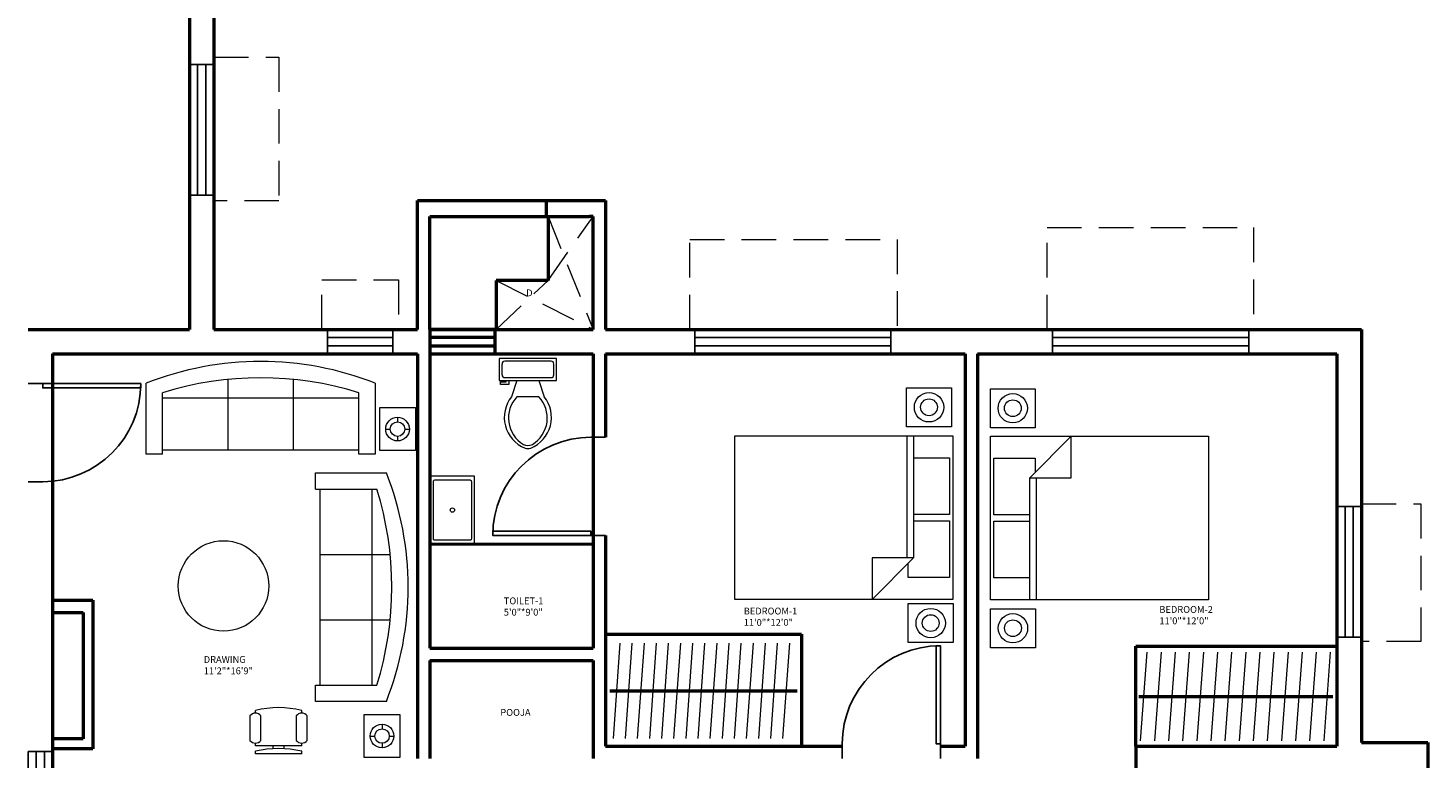
# Model space of a CAD drawing. Units: inches. Extents: x 291 to 2631, y 456 to 2623.
# Tile 11 of 22: x 2109 to 2623, y 774 to 1042. Entities that reach past the tile are written whole.
import ezdxf

# ---------------------------------------------------------------- set-up
doc = ezdxf.new("R2010")
doc.units = ezdxf.units.IN
doc.linetypes.add('DASHED', pattern=[19.05, 12.7, -6.35])
for name, color, linetype, lineweight in [('A-ANNO-TEXT', 3, 'Continuous', 25), ('A-AREA-IDEN', 7, 'Continuous', 25), ('A-DOOR', 3, 'Continuous', 25), ('A-FLOR-FIXT', 9, 'Continuous', 18), ('A-FLOR-OVHD', 1, 'DASHED', 18), ('A-FURN', 8, 'Continuous', 18), ('A-GLAZ', 4, 'Continuous', 25), ('A-WALL', 7, 'Continuous', 50)]:
    doc.layers.add(name, color=color, linetype=linetype, lineweight=lineweight)
doc.styles.get("Standard").update_dxf_attribs({"font": 'arial.ttf'})

# ---------------------------------------------------------------- blocks, each defined once
blk = doc.blocks.new('*U2')
for p, q in [((0, 0), (0, -6)), ((40, 0), (40, -6))]:
    blk.add_line(p, q)
blk.add_lwpolyline([(0, 0), (0, 40), (1.75, 40), (1.75, 0)], close=True)
blk.add_arc((0, 0), 40, 0, 90)
blk = doc.blocks.new('Sofa - Roundback 7 ft.')
for p, q in [((-12.00002, -32.4421), (-12.00003, -6.5971)), ((11.99997, -32.4421), (11.99998, -6.5971)), ((-36.000027, -34), (-36.000027, -11.4696)), ((-35.999844, -13.3819), (35.9998, -13.3819)), ((35.99998, -34), (35.99998, -11.4696)), ((-36.000027, -32.4421), (35.99998, -32.4421))]:
    blk.add_line(p, q)
for points in [[(-36.000027, -34), (-42.000027, -34), (-42.000027, -8)], [(41.99998, -8), (41.99998, -34), (35.99998, -34)]]:
    blk.add_lwpolyline(points)
for centre, radius, start, end in [((0, -114.25), 114.25, 68.43141, 111.5686), ((-0.00001, -127.1968), 121.1968, 72.72033, 107.2797)]:
    blk.add_arc(centre, radius, start, end)
blk = doc.blocks.new('Chair - Desk')
for p, q in [((-8.5, 0), (-8.5, -1)), ((-8.5, 0), (8.5, 0)), ((8.5, 0), (8.5, -1)), ((-10.5, -5), (-10.5, -14)), ((-8.5, -3), (-8.5, -4)), ((-8.5, -3), (8.5, -3)), ((-6.5, -14), (-6.5, -5)), ((-2, -3), (-2, -1.9355)), ((2, -1.9576), (2, -3)), ((6.5, -5), (6.5, -14)), ((8.5, -3), (8.5, -4)), ((10.5, -14), (10.5, -5)), ((-8.5, -15), (-8.5, -16)), ((8.5, -15), (8.5, -16))]:
    blk.add_line(p, q)
for centre, radius, start, end in [((-8.5, -6.5), 2.5, 36.8699, 143.1301), ((0, 34.625), 36.625, 256.5803, 283.4197), ((8.5, -6.5), 2.5, 36.8699, 143.1301), ((-8.5, -12.5), 2.5, 216.8699, 323.1301), ((8.5, -12.5), 2.5, 216.8699, 323.1301), ((0, 19.625), 36.625, 256.5803, 283.4197)]:
    blk.add_arc(centre, radius, start, end)
blk = doc.blocks.new('Toilet - top')
for p, q in [((9.5, -6), (9.5, -2)), ((-10, -8.5), (-8, -8.5)), ((-10, -9.5), (-10, -8.5)), ((-7, -9.5), (-10, -9.5)), ((-8, -8.5), (-8, -8)), ((-7, -8), (-7, -9.5)), ((-4, -8), (-6, -14)), ((4, -8), (6, -14)), ((4, -14), (-4, -14))]:
    blk.add_line(p, q)
blk.add_lwpolyline([(10.5, -8), (10.5, 0), (-10.5, 0), (-10.5, -8)], close=True)
for points in [[(-9.5, -2), (-9.5, -6)], [(8.5, -1), (-8.5, -1)], [(-8.5, -7), (8.5, -7)]]:
    blk.add_lwpolyline(points)
for centre, radius, start, end in [((-8.62, -1.88), 0.884, 81.8699, 188.1301), ((8.62, -1.88), 0.884, 351.8699, 98.1301), ((-8.62, -6.12), 0.884, 171.8699, 278.1301), ((8.62, -6.12), 0.884, 261.8699, 8.1301), ((3.52, -21.58), 12.17, 141.4691, 247.9714), ((4.2, -21.82), 11.33, 136.3677, 238.9468), ((-3.52, -21.58), 12.17, 292.0284, 38.5307), ((-4.2, -21.82), 11.33, 301.053, 43.6321), ((0, -27.88), 4, 245.7318, 294.2682), ((0, -29), 4, 254.8605, 285.1395)]:
    blk.add_arc(centre, radius, start, end)
blk = doc.blocks.new('Bed - Queen')
for p, q in [((0, -80.00003), (0, 0)), ((0, 0), (59.99999, 0)), ((59.99999, 0), (59.99999, -80.00003)), ((7.99999, -1.2), (28.79998, -1.2)), ((7.99999, -14.4), (7.99999, -1.2)), ((28.79998, -1.2), (28.79998, -14.4)), ((31.19999, -1.2), (51.99999, -1.2)), ((31.19999, -14.4), (31.19999, -1.2)), ((51.99999, -1.2), (51.99999, -16.4)), ((0, -14.4), (44.8, -14.4)), ((59.99999, -29.6), (44.8, -14.4)), ((44.8, -14.4), (44.8, -29.6)), ((44.8, -16.8), (0, -16.8)), ((51.99999, -16.4), (46.79936, -16.4)), ((44.8, -29.6), (59.99999, -29.6)), ((59.99999, -80.00003), (0, -80.00003))]:
    blk.add_line(p, q)
blk = doc.blocks.new('WIN-1800')
for p, q in [((0, 9), (72, 9)), ((0, 0), (0, 9)), ((0, 6), (72, 6)), ((72, 9), (72, 0)), ((72, 3), (0, 3)), ((72, 0), (0, 0))]:
    blk.add_line(p, q)
blk = doc.blocks.new('WIN-1200')
for p, q in [((0, 0), (0, 48)), ((0, 48), (9, 48)), ((3, 0), (3, 48)), ((6, 48), (6, 0)), ((9, 48), (9, 0)), ((9, 0), (0, 0))]:
    blk.add_line(p, q)
blk = doc.blocks.new('WIN-600')
for p, q in [((24, 9), (0, 9)), ((0, 9), (0, 0)), ((24, 6), (0, 6)), ((24, 0), (24, 9)), ((0, 3), (24, 3)), ((0, 0), (24, 0))]:
    blk.add_line(p, q)
blk = doc.blocks.new('LAMP-A')
for p, q in [((6.55, 12.25), (6.55, 10.56)), ((2.2, 7.9), (3.88, 7.9)), ((6.55, 5.24), (6.55, 3.56)), ((9.21, 7.9), (10.89, 7.9))]:
    blk.add_line(p, q)
blk.add_lwpolyline([(0, 15.8), (13.09, 15.8), (13.09, 0), (0, 0)], close=True)
for radius in [4.34, 2.66]:
    blk.add_circle((6.55, 7.9), radius)

msp = doc.modelspace()

# ---------------------------------------------------------------- linework, layer by layer
at = {"layer": 'A-FLOR-OVHD'}
for p, q in [((2177.21, 1030.97), (2201.09, 1030.97)), ((2201.09, 1030.97), (2201.09, 978.24)), ((2201.09, 978.24), (2177.21, 978.24)), ((2299.87, 972.51), (2316.47, 930.98)), ((2299.87, 948.94), (2316.47, 972.51)), ((2483.05, 930.98), (2483.05, 968.4)), ((2483.05, 968.4), (2558.88, 968.4)), ((2558.88, 968.4), (2558.88, 930.98)), ((2351.9, 930.98), (2351.9, 964.04)), ((2351.9, 964.04), (2428.07, 964.04)), ((2428.07, 964.04), (2428.07, 930.98)), ((2216.81, 930.98), (2216.81, 949.22)), ((2216.81, 949.22), (2244.97, 949.22)), ((2244.97, 949.22), (2244.97, 930.98)), ((2280.82, 948.94), (2316.47, 930.98)), ((2280.82, 930.98), (2299.87, 948.94)), ((2598.47, 866.98), (2620.33, 866.98)), ((2620.33, 866.98), (2620.33, 816.39)), ((2620.33, 816.39), (2598.47, 816.39))]:
    msp.add_line(p, q, dxfattribs=at)
at = {"layer": 'A-FURN'}
for p, q in [((2323.87, 780.85), (2326.34, 815.77)), ((2328.32, 780.85), (2330.78, 815.77)), ((2332.76, 780.85), (2335.23, 815.77)), ((2337.21, 780.85), (2339.68, 815.77)), ((2341.66, 780.85), (2344.12, 815.77)), ((2346.1, 780.85), (2348.57, 815.77)), ((2350.55, 780.85), (2353.02, 815.77)), ((2355, 780.85), (2357.46, 815.77)), ((2359.44, 780.85), (2361.91, 815.77)), ((2363.89, 780.85), (2366.35, 815.77)), ((2368.33, 780.85), (2370.8, 815.77)), ((2372.78, 780.85), (2375.25, 815.77)), ((2377.23, 780.85), (2379.69, 815.77)), ((2381.67, 780.85), (2384.14, 815.77)), ((2386.12, 780.85), (2388.59, 815.77)), ((2517.42, 779.97), (2519.86, 812.55)), ((2522.6, 779.97), (2525.04, 812.55)), ((2527.77, 779.97), (2530.22, 812.55)), ((2532.95, 779.97), (2535.4, 812.55)), ((2538.13, 779.97), (2540.57, 812.55)), ((2543.31, 779.97), (2545.75, 812.55)), ((2548.48, 779.97), (2550.93, 812.55)), ((2553.66, 779.97), (2556.11, 812.55)), ((2558.84, 779.97), (2561.28, 812.55)), ((2564.02, 779.97), (2566.46, 812.55)), ((2569.2, 779.97), (2571.64, 812.55)), ((2574.37, 779.97), (2576.82, 812.55)), ((2579.55, 779.97), (2581.99, 812.55)), ((2584.73, 779.97), (2587.17, 812.55))]:
    msp.add_line(p, q, dxfattribs=at)
for points in [[(2431.49, 909.56), (2447.97, 909.56), (2447.97, 895.26), (2431.49, 895.26)], [(2462.24, 909.21), (2478.72, 909.21), (2478.72, 894.91), (2462.24, 894.91)], [(2256.47, 852.14), (2272.82, 852.14), (2272.82, 877.08), (2256.47, 877.08)], [(2432.11, 830.34), (2448.59, 830.34), (2448.59, 816.04), (2432.11, 816.04)], [(2462.3, 828.43), (2478.78, 828.43), (2478.78, 814.13), (2462.3, 814.13)]]:
    msp.add_lwpolyline(points, close=True, dxfattribs=at)
msp.add_lwpolyline([(2258.32, 875.72), (2271.24, 875.72, -0.414214), (2271.74, 875.22), (2271.74, 854.12, -0.414214), (2271.24, 853.62), (2258.32, 853.62, -0.414214), (2257.82, 854.12), (2257.82, 875.22, -0.414214)], format="xyb", close=True, dxfattribs=at)
for centre, radius in [((2439.73, 902.41), 5.39), ((2439.73, 902.41), 3.08), ((2470.48, 902.06), 5.39), ((2470.48, 902.06), 3.08), ((2264.78, 864.67), 0.806), ((2180.72, 836.81), 16.61), ((2440.35, 823.19), 5.39), ((2440.35, 823.19), 3.08), ((2470.54, 821.28), 5.39), ((2470.54, 821.28), 3.08)]:
    msp.add_circle(centre, radius, dxfattribs=at)
at = {"layer": 'A-WALL'}
for p, q in [((2168.21, 1112.52), (2168.21, 930.98)), ((2177.21, 1112.52), (2177.21, 930.98)), ((2251.97, 930.98), (2251.97, 978.3)), ((2251.97, 978.3), (2320.97, 978.3)), ((2299.15, 978.3), (2299.15, 972.51)), ((2320.97, 978.3), (2320.97, 930.98)), ((2256.47, 930.98), (2256.47, 972.51)), ((2256.47, 972.51), (2314.97, 972.51)), ((2299.87, 972.51), (2299.87, 948.94)), ((2316.47, 972.51), (2314.97, 972.51)), ((2316.47, 930.98), (2316.47, 972.51)), ((2299.87, 948.94), (2280.82, 948.94)), ((2280.82, 948.94), (2280.82, 930.98)), ((2108.97, 930.98), (2168.21, 930.98)), ((2177.21, 930.98), (2251.97, 930.98)), ((2256.47, 930.98), (2256.47, 813.98)), ((2280.47, 930.98), (2256.47, 930.98)), ((2256.47, 930.98), (2256.47, 921.98)), ((2256.47, 930.98), (2316.47, 930.98)), ((2280.47, 921.98), (2280.47, 930.98)), ((2320.97, 930.98), (2598.47, 930.98)), ((2598.47, 930.98), (2598.47, 779.28)), ((2280.47, 927.98), (2256.47, 927.98)), ((2117.97, 921.98), (2251.97, 921.98)), ((2117.97, 921.98), (2117.97, 720.98)), ((2251.97, 921.98), (2251.97, 773.48)), ((2256.47, 924.98), (2280.47, 924.98)), ((2256.47, 921.98), (2280.47, 921.98)), ((2256.47, 921.98), (2316.47, 921.98)), ((2316.47, 921.98), (2316.47, 813.98)), ((2320.97, 921.98), (2320.97, 891.39)), ((2320.97, 921.98), (2452.97, 921.98)), ((2452.97, 921.98), (2452.97, 777.98)), ((2457.47, 921.98), (2457.47, 773.48)), ((2457.47, 921.98), (2589.47, 921.98)), ((2589.47, 921.98), (2589.47, 777.98)), ((2320.97, 855.39), (2320.97, 777.98)), ((2256.47, 852.14), (2316.47, 852.23)), ((2117.97, 831.6), (2132.79, 831.6)), ((2132.79, 831.6), (2132.79, 777.06)), ((2117.97, 827.07), (2129.19, 827.07)), ((2129.19, 827.07), (2129.19, 780.66)), ((2320.97, 819.07), (2392.97, 819.07)), ((2392.97, 819.07), (2392.97, 777.98)), ((2256.47, 813.98), (2316.47, 813.98)), ((2515.69, 777.98), (2515.69, 814.67)), ((2515.69, 814.67), (2589.47, 814.67)), ((2256.47, 809.48), (2316.47, 809.48)), ((2256.47, 809.48), (2256.47, 773.48)), ((2316.47, 809.48), (2316.47, 773.48)), ((2322.5, 798.31), (2391.31, 798.31)), ((2516.78, 796.26), (2587.92, 796.26)), ((2129.19, 780.66), (2117.97, 780.66)), ((2132.79, 777.06), (2117.97, 777.06)), ((2320.97, 777.98), (2407.89, 777.98)), ((2443.89, 777.98), (2452.97, 777.98)), ((2515.69, 777.98), (2515.69, 765.67)), ((2515.69, 777.98), (2589.47, 777.98)), ((2598.47, 779.28), (2621.78, 779.28)), ((2621.78, 779.28), (2622.9, 779.28)), ((2622.9, 779.28), (2622.9, 756.88))]:
    msp.add_line(p, q, dxfattribs=at)

# ---------------------------------------------------------------- block references
at = {"layer": 'A-DOOR', "xscale": 0.9, "yscale": 0.9, "zscale": 0.9}
for p, rotation in [((2114.37, 911.1), 270), ((2315.57, 855.39), 90)]:
    msp.add_blockref('*U2', p, dxfattribs=dict(at, rotation=rotation))
at = {"layer": 'A-DOOR', "xscale": -0.9, "yscale": 0.9, "zscale": 0.9}
msp.add_blockref('*U2', (2443.89, 778.88), dxfattribs=at)
at = {"layer": 'A-FLOR-FIXT'}
msp.add_blockref('Toilet - top', (2292.47, 920.3), dxfattribs=at)
at = {"layer": 'A-FURN'}
for name, p in [('Sofa - Roundback 7 ft.', (2194.4, 919.24)), ('LAMP-A', (2238.07, 886.5)), ('LAMP-A', (2232.38, 773.82))]:
    msp.add_blockref(name, p, dxfattribs=at)
for name, p, rotation in [('Bed - Queen', (2448.46, 891.9), 270), ('Bed - Queen', (2462.29, 831.75), 90), ('Sofa - Roundback 7 ft.', (2248.52, 836.39), 270), ('Chair - Desk', (2200.94, 775.13), 180)]:
    msp.add_blockref(name, p, dxfattribs=dict(at, rotation=rotation))
at = {"layer": 'A-GLAZ', "rotation": 180}
for name, p in [('WIN-1200', (2177.21, 1028.26)), ('WIN-600', (2242.87, 930.98)), ('WIN-1200', (2598.47, 865.99)), ('WIN-1200', (2117.97, 776.04))]:
    msp.add_blockref(name, p, dxfattribs=at)
at = {"layer": 'A-GLAZ'}
for p in [(2353.72, 921.98), (2485.08, 921.98)]:
    msp.add_blockref('WIN-1800', p, dxfattribs=at)

# ---------------------------------------------------------------- texts
at = {"layer": 'A-ANNO-TEXT', "insert": (2291.85, 945.68), "char_height": 2.5, "attachment_point": 1}
msp.add_mtext_dynamic_manual_height_columns('D', width=2.4589, gutter_width=12.5, heights=[0], dxfattribs=at)
at = {"layer": 'A-AREA-IDEN', "char_height": 2.5, "attachment_point": 1}
for s, width, insert in [('TOILET-1\\P5\'0"*9\'0"', 43.3452, (2283.63, 832.59)), ('BEDROOM-1\\P11\'0"*12\'0"', 19.9459, (2371.71, 828.84)), ('BEDROOM-2\\P11\'0"*12\'0"', 42.0634, (2524.28, 829.43)), ('DRAWING\\P11\'2"*16\'9"', 48.9751, (2173.48, 811.07)), ('POOJA', 33.1994, (2282.35, 791.63))]:
    msp.add_mtext_dynamic_manual_height_columns(s, width=width, gutter_width=12.5, heights=[0], dxfattribs=dict(at, insert=insert))

doc.saveas('drawing.dxf')
